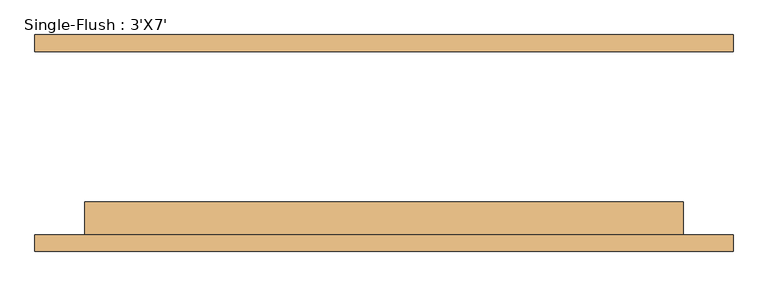
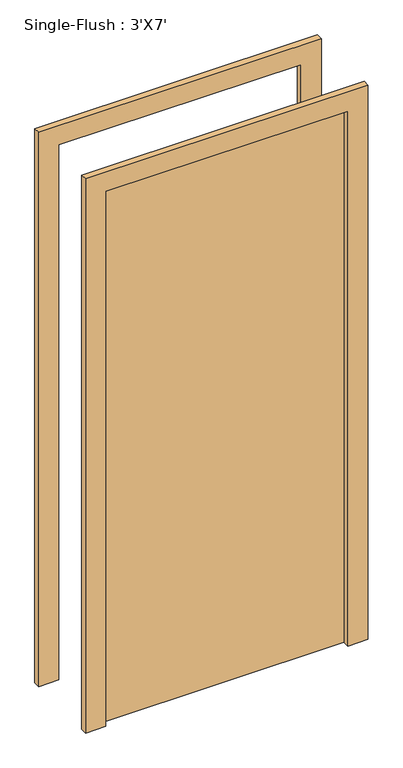
"""IFC4 building model written with IfcOpenShell, lengths in millimetres: door geometry, Single-Flush : 3'X7'."""

from ifc_helpers import new_model, si_unit, frame, origin, origin_with_axes, place, context, project, spatial, polyline, outline, extrude, source, transform, mapped, element, save


def single_flush_3_x7_4f727f60(model_context):
    return source(origin(), model_context, "Body", "SweptSolid", [
        extrude(outline(polyline([(2209.8, -533.4), (0.0, -533.4), (0.0, -457.2), (2133.6, -457.2), (2133.6, 457.2), (0.0, 457.2), (0.0, 533.4), (2209.8, 533.4), (2209.8, -533.4)])), frame((0.0, -165.8, 0.0), z_axis=(0.0, 1.0, 0.0), x_axis=(0.0, 0.0, 1.0)), (0.0, 0.0, 1.0), 25.4),
        extrude(outline(polyline([(2209.8, 533.4), (2209.8, -533.4), (0.0, -533.4), (0.0, -457.2), (2133.6, -457.2), (2133.6, 457.2), (0.0, 457.2), (0.0, 533.4), (2209.8, 533.4)])), frame((0.0, 140.4, 0.0), z_axis=(0.0, 1.0, 0.0), x_axis=(0.0, 0.0, 1.0)), (0.0, 0.0, 1.0), 25.4),
        extrude(outline(polyline([(457.2, -89.6), (457.2, -140.4), (-457.2, -140.4), (-457.2, -89.6), (457.2, -89.6)])), origin_with_axes(), (0.0, 0.0, 1.0), 2133.6),
    ])


if __name__ == "__main__":
    model = new_model("IFC4")
    model_context = context("Model", 3, world=origin())
    ifc_project = project(units=[si_unit("LENGTHUNIT", "METRE", prefix="MILLI")], contexts=[model_context])
    site = spatial("IfcSite", under=ifc_project)
    building = spatial("IfcBuilding", under=site)
    placement = place(None, origin())
    single_flush_3_x7_shape = single_flush_3_x7_4f727f60(model_context)
    element("IfcDoor", 1, ObjectType="Single-Flush : 3'X7'", at=placement, inside=building, context=model_context, shape_type="MappedRepresentation", body=[
        mapped(single_flush_3_x7_shape, transform((0.0, 0.0, 0.0), x_axis=(1.0, 0.0, 0.0), y_axis=(0.0, 1.0, 0.0), z_axis=(0.0, 0.0, 1.0))),
    ])
    save(model, "model.ifc")

# Revit data of these elements
# Type "Single-Flush : 3'X7'"
#   Type Mark = "10"
#   Assembly Code = "C1020"
#   Thickness = 0' - 2"
#   Height = 7' - 0"
#   Trim Projection Ext = 0' - 1"
#   Trim Projection Int = 0' - 1"
#   Trim Width = 0' - 3"
#   Width = 3' - 0"
#   Door Material = Door - Panel
#   Frame Material = Door - Frame
#   Function = (empty or 0)
#   Wall Closure = (empty or 0)
# Element 1 (IfcDoor, "Single-Flush : 3'X7'")
#   Materials on its faces: "Door - Frame", "Door - Panel"
# Materials
#   "Door - Panel": class "Wood", colour RGB 114 82 51, transparency 0
#   "Door - Frame": colour RGB 153 76 43, transparency 0
